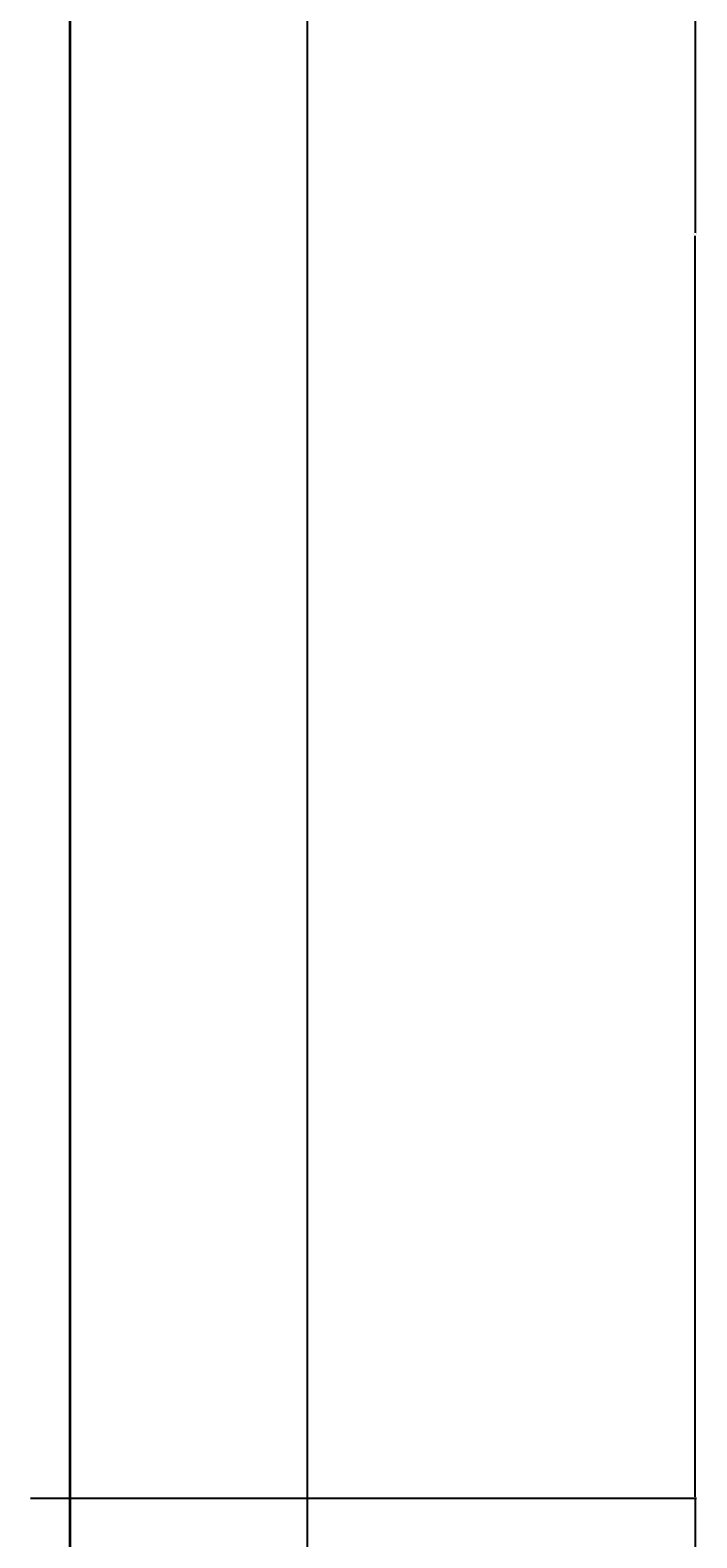
# Model space of a CAD drawing. Units: inches. Extents: x 3731 to 4318, y 1310 to 2388.
# Tile 48 of 57: x 4234 to 4318, y 1938 to 2129. Entities that reach past the tile are written whole.
import ezdxf

# ---------------------------------------------------------------- set-up
doc = ezdxf.new("R2010")
doc.units = ezdxf.units.IN
doc.layers.add('A-ANNO-DIMS', color=2, linetype='Continuous', lineweight=18)
doc.layers.add('A-WALL', color=7, linetype='Continuous', lineweight=35)
doc.styles.get("Standard").update_dxf_attribs({"font": 'arial.ttf'})
doc.dimstyles.get("Standard").update_dxf_attribs({"dimtxt": 0.18, "dimasz": 0.18, "dimexe": 0.18, "dimexo": 0.0625, "dimgap": 0.09, "dimtad": 0, "dimtih": 1, "dimtoh": 1, "dimdec": 4, "dimzin": 0, "dimdsep": 46, "dimtxsty": 'Standard', "dimcen": 0.09, "dimadec": 0, "dimazin": 0, "dimtfac": 1, "dimtdec": 4, "dimtofl": 0, "dimtmove": 0, "dimatfit": 3, "dimfxl": 1, "dimtolj": 1, "dimtzin": 0, "dimarcsym": 0})

# ---------------------------------------------------------------- blocks, each defined once
blk = doc.blocks.new('*D38')
at = {"layer": 'A-ANNO-DIMS', "color": 0, "lineweight": -2, "transparency": 16777216}
for p, q in [((4103.27, 2262.38), (4318.34, 2262.38)), ((4318.16, 2262.2), (4318.16, 2103.06)), ((4318.16, 1943.56), (4318.16, 2102.7)), ((4234.27, 1943.38), (4318.34, 1943.38))]:
    blk.add_line(p, q, dxfattribs=at)
at = {"layer": 'A-ANNO-DIMS', "color": 0, "transparency": 16777216}
for points in [[(4318.13, 2262.2), (4318.19, 2262.2), (4318.16, 2262.38)], [(4318.13, 1943.56), (4318.19, 1943.56), (4318.16, 1943.38)]]:
    blk.add_solid(points, dxfattribs=at)
at = {"layer": 'Defpoints', "color": 0, "transparency": 16777216}
for p in [(4103.21, 2262.38), (4318.16, 2262.38), (4234.21, 1943.38)]:
    blk.add_point(p, dxfattribs=at)
at = {"layer": 'A-ANNO-DIMS', "color": 0, "transparency": 16777216, "insert": (4318.16, 2102.88), "char_height": 0.18, "attachment_point": 5}
blk.add_mtext('\\A1;319', dxfattribs=at)
blk = doc.blocks.new('*D39')
at = {"layer": 'A-ANNO-DIMS', "color": 0, "lineweight": -2, "transparency": 16777216}
for p, q in [((4234.27, 1943.38), (4318.34, 1943.38)), ((4318.16, 1943.2), (4318.16, 1896.56)), ((4318.16, 1849.56), (4318.16, 1896.2)), ((4234.27, 1849.38), (4318.34, 1849.38))]:
    blk.add_line(p, q, dxfattribs=at)
at = {"layer": 'A-ANNO-DIMS', "color": 0, "transparency": 16777216}
for points in [[(4318.13, 1943.2), (4318.19, 1943.2), (4318.16, 1943.38)], [(4318.13, 1849.56), (4318.19, 1849.56), (4318.16, 1849.38)]]:
    blk.add_solid(points, dxfattribs=at)
at = {"layer": 'Defpoints', "color": 0, "transparency": 16777216}
for p in [(4234.21, 1943.38), (4318.16, 1943.38), (4234.21, 1849.38)]:
    blk.add_point(p, dxfattribs=at)
at = {"layer": 'A-ANNO-DIMS', "color": 0, "transparency": 16777216, "insert": (4318.16, 1896.38), "char_height": 0.18, "attachment_point": 5}
blk.add_mtext('\\A1;94', dxfattribs=at)
blk = doc.blocks.new('*D51')
at = {"layer": 'A-ANNO-DIMS', "color": 0, "lineweight": -2, "transparency": 16777216}
for p, q in [((4239.21, 1708.44), (4239.21, 2387.51)), ((4239.39, 2387.33), (4253.99, 2387.33)), ((4269.03, 2387.33), (4254.43, 2387.33)), ((4269.21, 1708.44), (4269.21, 2387.51))]:
    blk.add_line(p, q, dxfattribs=at)
at = {"layer": 'A-ANNO-DIMS', "color": 0, "transparency": 16777216}
for points in [[(4239.39, 2387.36), (4239.39, 2387.3), (4239.21, 2387.33)], [(4269.03, 2387.36), (4269.03, 2387.3), (4269.21, 2387.33)]]:
    blk.add_solid(points, dxfattribs=at)
at = {"layer": 'Defpoints', "color": 0, "transparency": 16777216}
for p in [(4269.21, 2387.33), (4239.21, 1708.38), (4269.21, 1708.38)]:
    blk.add_point(p, dxfattribs=at)
at = {"layer": 'A-ANNO-DIMS', "color": 0, "transparency": 16777216, "insert": (4254.21, 2387.33), "char_height": 0.18, "attachment_point": 5}
blk.add_mtext('\\A1;30', dxfattribs=at)

msp = doc.modelspace()

# ---------------------------------------------------------------- linework, layer by layer
at = {"layer": 'A-WALL'}
msp.add_line((4239.21, 2338.38), (4239.21, 1708.38), dxfattribs=at)

# ---------------------------------------------------------------- dimensions: what is measured, and where the dimension line sits
at = {"layer": 'A-ANNO-DIMS'}
dim = msp.add_linear_dim(base=(4269.21, 2387.33), p1=(4239.21, 1708.38), p2=(4269.21, 1708.38), dimstyle='Standard', override={"dimdec": 0, "dimlfac": 1, "dimrnd": 0, "dimzin": 0, "dimdsep": 46, "dimlunit": 2}, dxfattribs=at)
dim.commit()
dim.dimension.update_dxf_attribs({"geometry": '*D51', "text_midpoint": (4254.21, 2387.33)})
for base, p1, p2, picture, middle in [((4318.16, 2262.38), (4234.21, 1943.38), (4103.21, 2262.38), '*D38', (4318.16, 2102.88)), ((4318.16, 1943.38), (4234.21, 1849.38), (4234.21, 1943.38), '*D39', (4318.16, 1896.38))]:
    dim = msp.add_linear_dim(base=base, p1=p1, p2=p2, angle=90, dimstyle='Standard', override={"dimdec": 0, "dimlfac": 1, "dimrnd": 0, "dimzin": 0, "dimdsep": 46, "dimlunit": 2}, dxfattribs=at)
    dim.commit()
    dim.dimension.update_dxf_attribs({"geometry": picture, "text_midpoint": middle})

doc.saveas('drawing.dxf')
